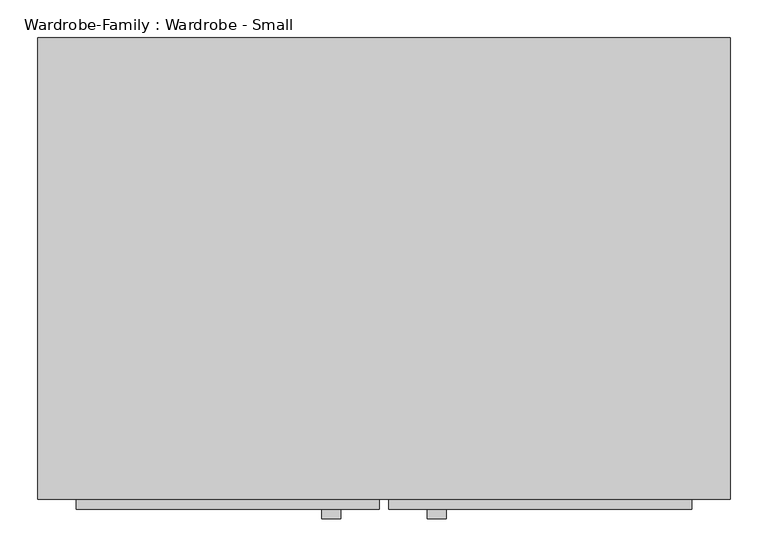
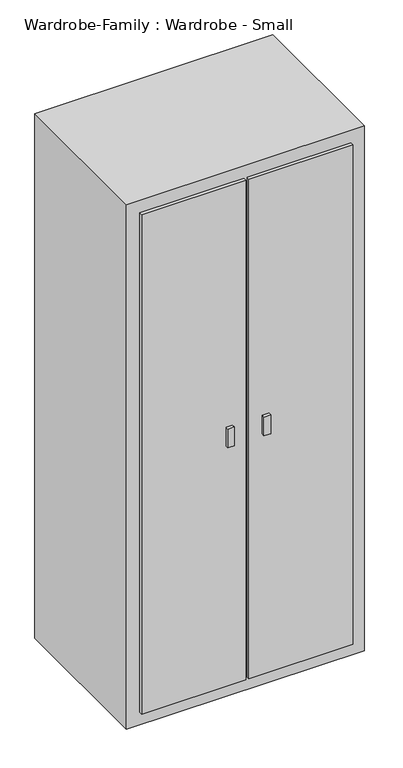
"""IFC4 building model written with IfcOpenShell, lengths in millimetres: furniture geometry, Wardrobe-Family : Wardrobe - Small."""

from ifc_helpers import new_model, si_unit, frame, origin, origin_with_axes, place, context, project, spatial, polyline, outline, extrude, source, transform, mapped, element, save


def wardrobe_family_wardrobe_small_46214fc7(model_context):
    return source(origin(), model_context, "Body", "SweptSolid", [
        extrude(outline(polyline([(457.2, -304.8), (-457.2, -304.8), (-457.2, 304.8), (457.2, 304.8), (457.2, -304.8)])), origin_with_axes(), (0.0, 0.0, 1.0), 2133.6),
        extrude(outline(polyline([(-6.35, -304.8), (-6.35, -317.5), (-406.4, -317.5), (-406.4, -304.8), (-6.35, -304.8)])), frame((0.0, 0.0, 50.8), z_axis=(0.0, 0.0, 1.0), x_axis=(1.0, 0.0, 0.0)), (0.0, 0.0, 1.0), 2032.0),
        extrude(outline(polyline([(406.4, -317.5), (6.35, -317.5), (6.35, -304.8), (406.4, -304.8), (406.4, -317.5)])), frame((0.0, 0.0, 50.8), z_axis=(0.0, 0.0, 1.0), x_axis=(1.0, 0.0, 0.0)), (0.0, 0.0, 1.0), 2032.0),
        extrude(outline(polyline([(-57.1834134, -317.5), (-57.1834134, -330.2), (-82.3387685, -330.2), (-82.3387685, -317.5), (-57.1834134, -317.5)])), frame((0.0, 0.0, 1028.7), z_axis=(0.0, 0.0, 1.0), x_axis=(1.0, 0.0, 0.0)), (0.0, 0.0, 1.0), 76.2),
        extrude(outline(polyline([(57.1834134, -330.2), (57.1834134, -317.5), (82.3387685, -317.5), (82.3387685, -330.2), (57.1834134, -330.2)])), frame((0.0, 0.0, 1028.7), z_axis=(0.0, 0.0, 1.0), x_axis=(1.0, 0.0, 0.0)), (0.0, 0.0, 1.0), 76.2),
    ])


if __name__ == "__main__":
    model = new_model("IFC4")
    model_context = context("Model", 3, world=origin())
    ifc_project = project(units=[si_unit("LENGTHUNIT", "METRE", prefix="MILLI")], contexts=[model_context])
    site = spatial("IfcSite", under=ifc_project)
    building = spatial("IfcBuilding", under=site)
    placement = place(None, origin())
    wardrobe_family_wardrobe_small_shape = wardrobe_family_wardrobe_small_46214fc7(model_context)
    element("IfcFurniture", 1, ObjectType="Wardrobe-Family : Wardrobe - Small", at=placement, inside=building, context=model_context, shape_type="MappedRepresentation", body=[
        mapped(wardrobe_family_wardrobe_small_shape, transform((0.0, 0.0, 0.0), x_axis=(1.0, 0.0, 0.0), y_axis=(0.0, 1.0, 0.0), z_axis=(0.0, 0.0, 1.0))),
    ])
    save(model, "model.ifc")

# Revit data of these elements
# Type "Wardrobe-Family : Wardrobe - Small"
#   Width = 2.0 ft
#   Length = 3.0 ft
#   Default Elevation = 0
# Element 1 (IfcFurniture, "Wardrobe-Family : Wardrobe - Small")
#   Materials on its faces: "Wood Material", "Steel Handle"
# Materials
#   "Wood Material": class "Generic", colour RGB 128 72 40, transparency 0, Cost = 0
#   "Steel Handle": class "Generic", colour RGB 206 211 212, transparency 0, Cost = 0
